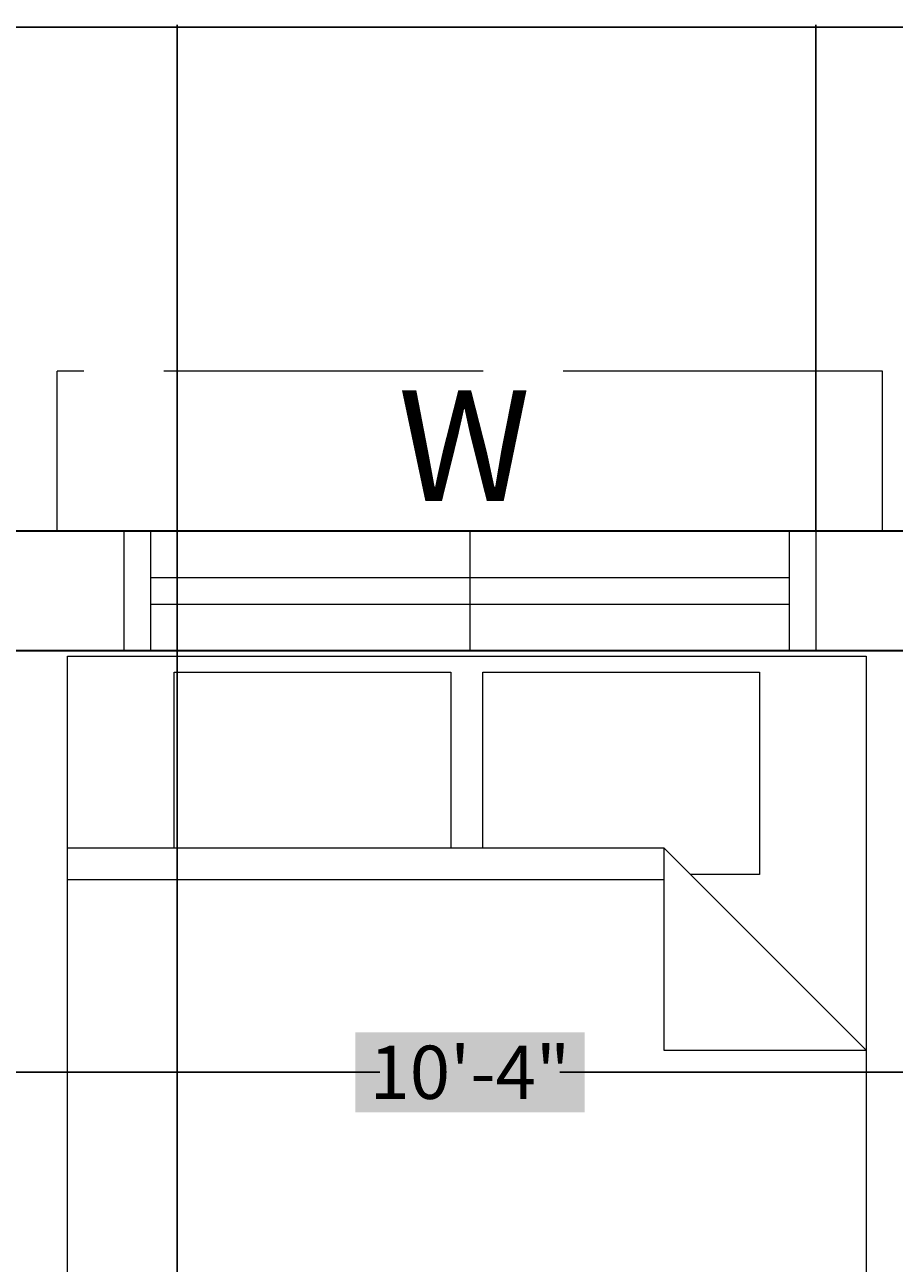
# Model space of a CAD drawing. Units: inches. Extents: x -128 to 854, y -395 to 398.
# Tile 48 of 61: x 209 to 275, y 294 to 387. Entities that reach past the tile are written whole.
import ezdxf

# ---------------------------------------------------------------- set-up
doc = ezdxf.new("R2010")
doc.units = ezdxf.units.IN
doc.header["$MEASUREMENT"] = 0
doc.linetypes.add('ACAD_ISO02W100', pattern=[15, 12, -3])
for name, color, linetype, lineweight in [('A-ANNO-DIMS', 2, 'Continuous', 18), ('A-ANNO-TEXT', 2, 'Continuous', 18), ('A-FURN', 8, 'Continuous', 18), ('A-GLAZ', 220, 'Continuous', 18), ('A-GLAZ-OVHD', 220, 'ACAD_ISO02W100', 13), ('A-WALL', 4, 'Continuous', 35)]:
    doc.layers.add(name, color=color, linetype=linetype, lineweight=lineweight)
doc.styles.get("Standard").update_dxf_attribs({"font": 'arial.ttf'})
doc.dimstyles.get("Standard").update_dxf_attribs({"dimtxt": 0.18, "dimasz": 0.18, "dimexe": 0.18, "dimexo": 0.0625, "dimgap": 0.09, "dimtad": 0, "dimtih": 1, "dimtoh": 1, "dimdec": 1, "dimzin": 0, "dimdsep": 46, "dimlunit": 4, "dimtxsty": 'Standard', "dimcen": 0.09, "dimclrd": 1, "dimclre": 2, "dimclrt": 6, "dimadec": 0, "dimazin": 0, "dimtfac": 1, "dimtdec": 1, "dimtofl": 0, "dimtmove": 0, "dimatfit": 3, "dimfxl": 1, "dimtfill": 2, "dimtfillclr": 3, "dimtolj": 1, "dimtzin": 0, "dimarcsym": 0})

# ---------------------------------------------------------------- blocks, each defined once
blk = doc.blocks.new('Bed - Queen')
for p, q in [((0, -80.00003), (0, 0)), ((0, 0), (59.99999, 0)), ((59.99999, 0), (59.99999, -80.00003)), ((7.99999, -1.2), (28.79998, -1.2)), ((7.99999, -14.4), (7.99999, -1.2)), ((28.79998, -1.2), (28.79998, -14.4)), ((31.19999, -1.2), (51.99999, -1.2)), ((31.19999, -14.4), (31.19999, -1.2)), ((51.99999, -1.2), (51.99999, -16.4)), ((0, -14.4), (44.8, -14.4)), ((59.99999, -29.6), (44.8, -14.4)), ((44.8, -14.4), (44.8, -29.6)), ((51.99999, -16.4), (46.79936, -16.4)), ((44.8, -16.8), (0, -16.8)), ((44.8, -29.6), (59.99999, -29.6)), ((59.99999, -80.00003), (0, -80.00003))]:
    blk.add_line(p, q)
blk = doc.blocks.new('*D52')
at = {"layer": 'A-ANNO-DIMS', "color": 0, "lineweight": -2, "transparency": 16777216}
for p, q in [((180.873, 339.678), (180.873, 307.9)), ((304.873, 339.678), (304.873, 307.9)), ((185.873, 308.08), (236.101, 308.08)), ((299.873, 308.08), (249.645, 308.08))]:
    blk.add_line(p, q, dxfattribs=at)
at = {"layer": 'A-ANNO-DIMS', "color": 0, "transparency": 16777216}
for points in [[(185.873, 308.913), (185.873, 307.247), (180.873, 308.08)], [(299.873, 308.913), (299.873, 307.247), (304.873, 308.08)]]:
    blk.add_solid(points, dxfattribs=at)
at = {"layer": 'Defpoints', "color": 0, "transparency": 16777216}
for p in [(180.873, 339.741), (304.873, 339.741), (304.873, 308.08)]:
    blk.add_point(p, dxfattribs=at)
at = {"layer": 'A-ANNO-DIMS', "color": 0, "transparency": 16777216, "insert": (242.873, 308.08), "char_height": 4, "attachment_point": 5, "bg_fill": 1, "box_fill_scale": 1.25, "bg_fill_color": 3, "bg_fill_transparency": 0}
blk.add_mtext('\\A1;10\'-4"', dxfattribs=at)
blk = doc.blocks.new('WIN-48IN')
for p, q in [((9, 52), (0, 52)), ((9, 50), (0, 50)), ((3.5, 50), (3.5, 2)), ((5.5, 50), (5.5, 2)), ((9, 26), (0, 26)), ((9, 2), (0, 2)), ((9, 0), (0, 0))]:
    blk.add_line(p, q)
blk = doc.blocks.new('SHADE-48IN')
at = {"ltscale": 2}
for p, q in [((12, 62), (0, 62)), ((0, 0), (0, 62)), ((12, 57), (12, 62)), ((12, 5), (12, 0)), ((12, 0), (0, 0))]:
    blk.add_line(p, q, dxfattribs=at)
blk = doc.blocks.new('*D97')
at = {"layer": 'A-ANNO-DIMS', "color": 2, "lineweight": -2, "transparency": 16777216}
for p, q in [((-50.127, 348.803), (-50.127, 386.743)), ((313.873, 348.803), (313.873, 386.743))]:
    blk.add_line(p, q, dxfattribs=at)
at = {"layer": 'A-ANNO-DIMS', "color": 1, "lineweight": -2, "transparency": 16777216}
for p, q in [((-49.947, 386.563), (131.474, 386.563)), ((313.693, 386.563), (132.272, 386.563))]:
    blk.add_line(p, q, dxfattribs=at)
at = {"layer": 'A-ANNO-DIMS', "color": 1, "transparency": 16777216}
for points in [[(-49.947, 386.593), (-49.947, 386.533), (-50.127, 386.563)], [(313.693, 386.593), (313.693, 386.533), (313.873, 386.563)]]:
    blk.add_solid(points, dxfattribs=at)
at = {"layer": 'Defpoints', "color": 0, "transparency": 16777216}
for p in [(313.873, 386.563), (-50.127, 348.741), (313.873, 348.741)]:
    blk.add_point(p, dxfattribs=at)
at = {"layer": 'A-ANNO-DIMS', "color": 6, "transparency": 16777216, "insert": (131.873, 386.563), "char_height": 0.18, "attachment_point": 5, "bg_fill": 1, "box_fill_scale": 1.25, "bg_fill_color": 3, "bg_fill_transparency": 0}
blk.add_mtext('\\A1;30\'-4"', dxfattribs=at)
blk = doc.blocks.new('*D101')
at = {"layer": 'A-ANNO-DIMS', "color": 2, "lineweight": -2, "transparency": 16777216}
for p, q in [((180.873, 186.803), (180.873, 386.743)), ((220.873, 186.803), (220.873, 386.743))]:
    blk.add_line(p, q, dxfattribs=at)
at = {"layer": 'A-ANNO-DIMS', "color": 1, "lineweight": -2, "transparency": 16777216}
for p, q in [((181.053, 386.563), (200.544, 386.563)), ((220.693, 386.563), (201.202, 386.563))]:
    blk.add_line(p, q, dxfattribs=at)
at = {"layer": 'A-ANNO-DIMS', "color": 1, "transparency": 16777216}
for points in [[(181.053, 386.593), (181.053, 386.533), (180.873, 386.563)], [(220.693, 386.593), (220.693, 386.533), (220.873, 386.563)]]:
    blk.add_solid(points, dxfattribs=at)
at = {"layer": 'Defpoints', "color": 0, "transparency": 16777216}
for p in [(220.873, 386.563), (180.873, 186.741), (220.873, 186.741)]:
    blk.add_point(p, dxfattribs=at)
at = {"layer": 'A-ANNO-DIMS', "color": 6, "transparency": 16777216, "insert": (200.873, 386.563), "char_height": 0.18, "attachment_point": 5, "bg_fill": 1, "box_fill_scale": 1.25, "bg_fill_color": 3, "bg_fill_transparency": 0}
blk.add_mtext('\\A1;3\'-4"', dxfattribs=at)
blk = doc.blocks.new('*D105')
at = {"layer": 'A-ANNO-DIMS', "color": 2, "lineweight": -2, "transparency": 16777216}
for p, q in [((268.873, 348.803), (268.873, 386.743)), ((313.873, 348.803), (313.873, 386.743))]:
    blk.add_line(p, q, dxfattribs=at)
at = {"layer": 'A-ANNO-DIMS', "color": 1, "lineweight": -2, "transparency": 16777216}
for p, q in [((269.053, 386.563), (291.044, 386.563)), ((313.693, 386.563), (291.702, 386.563))]:
    blk.add_line(p, q, dxfattribs=at)
at = {"layer": 'A-ANNO-DIMS', "color": 1, "transparency": 16777216}
for points in [[(269.053, 386.593), (269.053, 386.533), (268.873, 386.563)], [(313.693, 386.593), (313.693, 386.533), (313.873, 386.563)]]:
    blk.add_solid(points, dxfattribs=at)
at = {"layer": 'Defpoints', "color": 0, "transparency": 16777216}
for p in [(268.873, 386.563), (268.873, 348.741), (313.873, 348.741)]:
    blk.add_point(p, dxfattribs=at)
at = {"layer": 'A-ANNO-DIMS', "color": 6, "transparency": 16777216, "insert": (291.373, 386.563), "char_height": 0.18, "attachment_point": 5, "bg_fill": 1, "box_fill_scale": 1.25, "bg_fill_color": 3, "bg_fill_transparency": 0}
blk.add_mtext('\\A1;3\'-9"', dxfattribs=at)

msp = doc.modelspace()

# ---------------------------------------------------------------- linework, layer by layer
at = {"layer": 'A-WALL'}
for p, q in [((180.873, 348.741), (313.873, 348.741)), ((180.873, 339.741), (304.873, 339.741))]:
    msp.add_line(p, q, dxfattribs=at)

# ---------------------------------------------------------------- block references
at = {"layer": 'A-FURN'}
msp.add_blockref('Bed - Queen', (212.644, 339.338), dxfattribs=at)
at = {"layer": 'A-GLAZ', "rotation": 90.00000000000006}
msp.add_blockref('WIN-48IN', (268.873, 339.741), dxfattribs=at)
at = {"layer": 'A-GLAZ-OVHD', "extrusion": (0, 0, -1), "zscale": -1, "rotation": 270}
msp.add_blockref('SHADE-48IN', (-273.873, 360.741), dxfattribs=at)

# ---------------------------------------------------------------- texts
at = {"layer": 'A-ANNO-TEXT'}
msp.add_text('W', height=8.314, dxfattribs=at).set_placement((237.477, 350.979))

# ---------------------------------------------------------------- dimensions: what is measured, and where the dimension line sits
at = {"layer": 'A-ANNO-DIMS'}
for base, p1, p2, override, picture, middle in [((313.873, 386.563), (-50.127, 348.741), (313.873, 348.741), {"dimdec": 1, "dimlfac": 1, "dimrnd": 0, "dimzin": 1, "dimdsep": 46, "dimlunit": 4, "dimfrac": 2}, '*D97', (131.873, 386.563)), ((220.873, 386.563), (180.873, 186.741), (220.873, 186.741), {"dimdec": 1, "dimlfac": 1, "dimrnd": 0, "dimzin": 1, "dimdsep": 46, "dimlunit": 4, "dimfrac": 2}, '*D101', (200.873, 386.563)), ((268.873, 386.563), (313.873, 348.741), (268.873, 348.741), {"dimdec": 1, "dimlfac": 1, "dimrnd": 0, "dimzin": 1, "dimdsep": 46, "dimlunit": 4, "dimfrac": 2}, '*D105', (291.373, 386.563)), ((304.873, 308.08), (180.873, 339.741), (304.873, 339.741), {"dimtxt": 4, "dimasz": 5, "dimclrd": 0, "dimclre": 0, "dimclrt": 0}, '*D52', (242.873, 308.08))]:
    dim = msp.add_linear_dim(base=base, p1=p1, p2=p2, dimstyle='Standard', override=override, dxfattribs=at)
    dim.commit()
    dim.dimension.update_dxf_attribs({"geometry": picture, "text_midpoint": middle})

doc.saveas('drawing.dxf')
